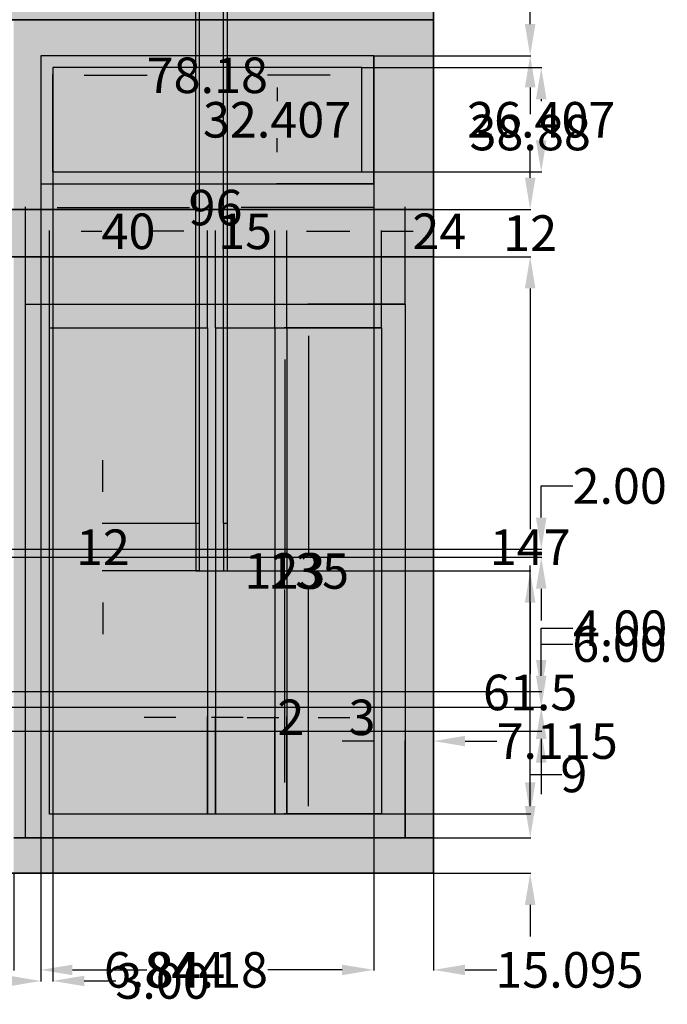
# Model space of a CAD drawing. Units: inches. Extents: x 207 to 609, y 30 to 576.
# Tile 2 of 4: x 445 to 609, y 30 to 279. Entities that reach past the tile are written whole.
import ezdxf

# ---------------------------------------------------------------- set-up
doc = ezdxf.new("R2010")
doc.units = ezdxf.units.IN
doc.header["$MEASUREMENT"] = 0
for name, color, linetype, lineweight in [('A-ANNO-DIMS', 2, 'Continuous', 18), ('A-DOOR', 3, 'Continuous', 25), ('A-ELEV', 7, 'Continuous', 35), ('A-ELEV-PATT', 251, 'Continuous', 13), ('A-ELEV-PATT-WOOD', 19, 'Continuous', 13), ('A-GLAZ', 4, 'Continuous', 25), ('A-GLAZ-PATT', 49, 'Continuous', 13)]:
    doc.layers.add(name, color=color, linetype=linetype, lineweight=lineweight)
doc.styles.get("Standard").update_dxf_attribs({"font": 'arial.ttf'})
doc.dimstyles.get("Standard").update_dxf_attribs({"dimtxt": 9, "dimasz": 8, "dimexe": 0.18, "dimexo": 0.0625, "dimgap": 0.09, "dimtad": 0, "dimtih": 1, "dimtoh": 1, "dimdec": 0, "dimzin": 0, "dimdsep": 46, "dimlunit": 3, "dimtxsty": 'Standard', "dimcen": 0.09, "dimadec": 0, "dimazin": 0, "dimtfac": 1, "dimtdec": 0, "dimtofl": 0, "dimtmove": 0, "dimatfit": 3, "dimfxl": 1, "dimtolj": 1, "dimtzin": 0, "dimarcsym": 0})

# ---------------------------------------------------------------- blocks, each defined once
blk = doc.blocks.new('*D18')
at = {"layer": 'A-ANNO-DIMS', "color": 0, "lineweight": -2, "transparency": 16777216}
for p, q in [((574.15, 79.79), (574.15, 87.79)), ((574.15, 87.79), (582.15, 87.79)), ((549.76, 71.79), (574.33, 71.79)), ((549.76, 62.79), (574.33, 62.79)), ((574.15, 54.79), (574.15, 46.79))]:
    blk.add_line(p, q, dxfattribs=at)
at = {"layer": 'A-ANNO-DIMS', "color": 0, "transparency": 16777216}
for points in [[(572.81, 79.79), (575.48, 79.79), (574.15, 71.79)], [(572.81, 54.79), (575.48, 54.79), (574.15, 62.79)]]:
    blk.add_solid(points, dxfattribs=at)
at = {"layer": 'Defpoints', "color": 0, "transparency": 16777216}
for p in [(549.7, 71.79), (574.15, 71.79), (549.7, 62.79)]:
    blk.add_point(p, dxfattribs=at)
at = {"layer": 'A-ANNO-DIMS', "color": 0, "transparency": 16777216, "insert": (585.19, 87.79), "char_height": 9, "attachment_point": 5}
blk.add_mtext('\\A1;9', dxfattribs=at)
blk = doc.blocks.new('*D19')
at = {"layer": 'A-ANNO-DIMS', "color": 0, "lineweight": -2, "transparency": 16777216}
for p, q in [((549.76, 218.79), (574.33, 218.79)), ((574.15, 210.79), (574.15, 149.89)), ((574.15, 79.79), (574.15, 140.68)), ((549.76, 71.79), (574.33, 71.79))]:
    blk.add_line(p, q, dxfattribs=at)
at = {"layer": 'A-ANNO-DIMS', "color": 0, "transparency": 16777216}
for points in [[(572.81, 210.79), (575.48, 210.79), (574.15, 218.79)], [(572.81, 79.79), (575.48, 79.79), (574.15, 71.79)]]:
    blk.add_solid(points, dxfattribs=at)
at = {"layer": 'Defpoints', "color": 0, "transparency": 16777216}
for p in [(549.7, 218.79), (574.15, 218.79), (549.7, 71.79)]:
    blk.add_point(p, dxfattribs=at)
at = {"layer": 'A-ANNO-DIMS', "color": 0, "transparency": 16777216, "insert": (574.15, 145.29), "char_height": 9, "attachment_point": 5}
blk.add_mtext('\\A1;147', dxfattribs=at)
blk = doc.blocks.new('*D20')
at = {"layer": 'A-ANNO-DIMS', "color": 0, "lineweight": -2, "transparency": 16777216}
for p, q in [((574.15, 238.79), (574.15, 246.79)), ((549.76, 230.79), (574.33, 230.79)), ((549.76, 218.79), (574.33, 218.79)), ((574.15, 210.79), (574.15, 202.79))]:
    blk.add_line(p, q, dxfattribs=at)
at = {"layer": 'A-ANNO-DIMS', "color": 0, "transparency": 16777216}
for points in [[(572.81, 238.79), (575.48, 238.79), (574.15, 230.79)], [(572.81, 210.79), (575.48, 210.79), (574.15, 218.79)]]:
    blk.add_solid(points, dxfattribs=at)
at = {"layer": 'Defpoints', "color": 0, "transparency": 16777216}
for p in [(549.7, 230.79), (574.15, 230.79), (549.7, 218.79)]:
    blk.add_point(p, dxfattribs=at)
at = {"layer": 'A-ANNO-DIMS', "color": 0, "transparency": 16777216, "insert": (574.15, 224.79), "char_height": 9, "attachment_point": 5}
blk.add_mtext('\\A1;12', dxfattribs=at)
blk = doc.blocks.new('*D21')
at = {"layer": 'A-ANNO-DIMS', "color": 0, "lineweight": -2, "transparency": 16777216}
for p, q in [((534.66, 269.66), (574.33, 269.66)), ((574.15, 261.66), (574.15, 254.91)), ((574.15, 238.79), (574.15, 245.54)), ((549.76, 230.79), (574.33, 230.79))]:
    blk.add_line(p, q, dxfattribs=at)
at = {"layer": 'A-ANNO-DIMS', "color": 0, "transparency": 16777216}
for points in [[(572.81, 261.66), (575.48, 261.66), (574.15, 269.66)], [(572.81, 238.79), (575.48, 238.79), (574.15, 230.79)]]:
    blk.add_solid(points, dxfattribs=at)
at = {"layer": 'Defpoints', "color": 0, "transparency": 16777216}
for p in [(534.6, 269.66), (574.15, 269.66), (549.7, 230.79)]:
    blk.add_point(p, dxfattribs=at)
at = {"layer": 'A-ANNO-DIMS', "color": 0, "transparency": 16777216, "insert": (574.15, 250.23), "char_height": 9, "attachment_point": 5}
blk.add_mtext('\\A1;38.88', dxfattribs=at)
blk = doc.blocks.new('*D22')
at = {"layer": 'A-ANNO-DIMS', "color": 0, "lineweight": -2, "transparency": 16777216}
for p, q in [((549.76, 302.79), (574.33, 302.79)), ((574.15, 294.79), (574.15, 290.91)), ((574.15, 277.66), (574.15, 281.54)), ((534.66, 269.66), (574.33, 269.66))]:
    blk.add_line(p, q, dxfattribs=at)
at = {"layer": 'A-ANNO-DIMS', "color": 0, "transparency": 16777216}
for points in [[(572.81, 294.79), (575.48, 294.79), (574.15, 302.79)], [(572.81, 277.66), (575.48, 277.66), (574.15, 269.66)]]:
    blk.add_solid(points, dxfattribs=at)
at = {"layer": 'Defpoints', "color": 0, "transparency": 16777216}
for p in [(549.7, 302.79), (574.15, 302.79), (534.6, 269.66)]:
    blk.add_point(p, dxfattribs=at)
at = {"layer": 'A-ANNO-DIMS', "color": 0, "transparency": 16777216, "insert": (574.15, 286.23), "char_height": 9, "attachment_point": 5}
blk.add_mtext('\\A1;33.12', dxfattribs=at)
blk = doc.blocks.new('*D32')
at = {"layer": 'A-ANNO-DIMS', "color": 0, "lineweight": -2, "transparency": 16777216}
for p, q in [((450.42, 269.6), (450.42, 38.16)), ((443.58, 62.72), (443.58, 38.16)), ((435.58, 38.34), (427.58, 38.34)), ((458.42, 38.34), (466.42, 38.34))]:
    blk.add_line(p, q, dxfattribs=at)
at = {"layer": 'A-ANNO-DIMS', "color": 0, "transparency": 16777216}
for points in [[(435.58, 39.67), (435.58, 37), (443.58, 38.34)], [(458.42, 39.67), (458.42, 37), (450.42, 38.34)]]:
    blk.add_solid(points, dxfattribs=at)
at = {"layer": 'Defpoints', "color": 0, "transparency": 16777216}
for p in [(450.42, 269.66), (443.58, 62.79), (450.42, 38.34)]:
    blk.add_point(p, dxfattribs=at)
at = {"layer": 'A-ANNO-DIMS', "color": 0, "transparency": 16777216, "insert": (481.71, 38.34), "char_height": 9, "attachment_point": 5}
blk.add_mtext('\\A1;6.844', dxfattribs=at)
blk = doc.blocks.new('*D33')
at = {"layer": 'A-ANNO-DIMS', "color": 0, "lineweight": -2, "transparency": 16777216}
for p, q in [((450.42, 269.6), (450.42, 38.16)), ((534.6, 269.6), (534.6, 38.16)), ((458.42, 38.34), (477.22, 38.34)), ((526.6, 38.34), (507.8, 38.34))]:
    blk.add_line(p, q, dxfattribs=at)
at = {"layer": 'A-ANNO-DIMS', "color": 0, "transparency": 16777216}
for points in [[(458.42, 39.67), (458.42, 37), (450.42, 38.34)], [(526.6, 39.67), (526.6, 37), (534.6, 38.34)]]:
    blk.add_solid(points, dxfattribs=at)
at = {"layer": 'Defpoints', "color": 0, "transparency": 16777216}
for p in [(450.42, 269.66), (534.6, 269.66), (534.6, 38.34)]:
    blk.add_point(p, dxfattribs=at)
at = {"layer": 'A-ANNO-DIMS', "color": 0, "transparency": 16777216, "insert": (492.51, 38.34), "char_height": 9, "attachment_point": 5}
blk.add_mtext('\\A1;84.18', dxfattribs=at)
blk = doc.blocks.new('*D34')
at = {"layer": 'A-ANNO-DIMS', "color": 0, "lineweight": -2, "transparency": 16777216}
for p, q in [((534.6, 269.6), (534.6, 38.16)), ((549.7, 62.72), (549.7, 38.16)), ((526.6, 38.34), (518.6, 38.34)), ((557.7, 38.34), (565.7, 38.34))]:
    blk.add_line(p, q, dxfattribs=at)
at = {"layer": 'A-ANNO-DIMS', "color": 0, "transparency": 16777216}
for points in [[(526.6, 39.67), (526.6, 37), (534.6, 38.34)], [(557.7, 39.67), (557.7, 37), (549.7, 38.34)]]:
    blk.add_solid(points, dxfattribs=at)
at = {"layer": 'Defpoints', "color": 0, "transparency": 16777216}
for p in [(534.6, 269.66), (549.7, 62.79), (549.7, 38.34)]:
    blk.add_point(p, dxfattribs=at)
at = {"layer": 'A-ANNO-DIMS', "color": 0, "transparency": 16777216, "insert": (584.08, 38.34), "char_height": 9, "attachment_point": 5}
blk.add_mtext('\\A1;15.095', dxfattribs=at)
blk = doc.blocks.new('*D35')
at = {"layer": 'A-ANNO-DIMS', "color": 0, "lineweight": -2, "transparency": 16777216}
for p, q in [((446.58, 206.85), (446.58, 231.42)), ((454.58, 231.24), (488.05, 231.24)), ((534.58, 231.24), (501.11, 231.24)), ((542.58, 206.85), (542.58, 231.42))]:
    blk.add_line(p, q, dxfattribs=at)
at = {"layer": 'A-ANNO-DIMS', "color": 0, "transparency": 16777216}
for points in [[(454.58, 232.57), (454.58, 229.9), (446.58, 231.24)], [(534.58, 232.57), (534.58, 229.9), (542.58, 231.24)]]:
    blk.add_solid(points, dxfattribs=at)
at = {"layer": 'Defpoints', "color": 0, "transparency": 16777216}
for p in [(542.58, 231.24), (446.58, 206.79), (542.58, 206.79)]:
    blk.add_point(p, dxfattribs=at)
at = {"layer": 'A-ANNO-DIMS', "color": 0, "transparency": 16777216, "insert": (494.58, 231.24), "char_height": 9, "attachment_point": 5}
blk.add_mtext('\\A1;96', dxfattribs=at)
blk = doc.blocks.new('*D36')
at = {"layer": 'A-ANNO-DIMS', "color": 0, "lineweight": -2, "transparency": 16777216}
for p, q in [((534.58, 96.24), (526.58, 96.24)), ((542.58, 71.85), (542.58, 96.42)), ((549.7, 71.85), (549.7, 96.42)), ((557.7, 96.24), (565.7, 96.24))]:
    blk.add_line(p, q, dxfattribs=at)
at = {"layer": 'A-ANNO-DIMS', "color": 0, "transparency": 16777216}
for points in [[(534.58, 97.57), (534.58, 94.9), (542.58, 96.24)], [(557.7, 97.57), (557.7, 94.9), (549.7, 96.24)]]:
    blk.add_solid(points, dxfattribs=at)
at = {"layer": 'Defpoints', "color": 0, "transparency": 16777216}
for p in [(549.7, 96.24), (542.58, 71.79), (549.7, 71.79)]:
    blk.add_point(p, dxfattribs=at)
at = {"layer": 'A-ANNO-DIMS', "color": 0, "transparency": 16777216, "insert": (580.97, 96.24), "char_height": 9, "attachment_point": 5}
blk.add_mtext('\\A1;7.115', dxfattribs=at)
blk = doc.blocks.new('*D37')
at = {"layer": 'A-ANNO-DIMS', "color": 0, "lineweight": -2, "transparency": 16777216}
for p, q in [((534.54, 269.66), (509.97, 269.66)), ((510.15, 261.66), (510.15, 258.15)), ((510.15, 245.26), (510.15, 248.77)), ((534.54, 237.26), (509.97, 237.26))]:
    blk.add_line(p, q, dxfattribs=at)
at = {"layer": 'A-ANNO-DIMS', "color": 0, "transparency": 16777216}
for points in [[(508.82, 261.66), (511.48, 261.66), (510.15, 269.66)], [(508.82, 245.26), (511.48, 245.26), (510.15, 237.26)]]:
    blk.add_solid(points, dxfattribs=at)
at = {"layer": 'Defpoints', "color": 0, "transparency": 16777216}
for p in [(510.15, 269.66), (534.6, 269.66), (534.6, 237.26)]:
    blk.add_point(p, dxfattribs=at)
at = {"layer": 'A-ANNO-DIMS', "color": 0, "transparency": 16777216, "insert": (510.15, 253.46), "char_height": 9, "attachment_point": 5}
blk.add_mtext('\\A1;32.407', dxfattribs=at)
blk = doc.blocks.new('*D38')
at = {"layer": 'A-ANNO-DIMS', "color": 0, "lineweight": -2, "transparency": 16777216}
for p, q in [((453.42, 240.32), (453.42, 264.89)), ((461.42, 264.71), (477.27, 264.71)), ((523.6, 264.71), (507.76, 264.71)), ((531.6, 240.32), (531.6, 264.89))]:
    blk.add_line(p, q, dxfattribs=at)
at = {"layer": 'A-ANNO-DIMS', "color": 0, "transparency": 16777216}
for points in [[(461.42, 266.04), (461.42, 263.37), (453.42, 264.71)], [(523.6, 266.04), (523.6, 263.37), (531.6, 264.71)]]:
    blk.add_solid(points, dxfattribs=at)
at = {"layer": 'Defpoints', "color": 0, "transparency": 16777216}
for p in [(531.6, 264.71), (453.42, 240.26), (531.6, 240.26)]:
    blk.add_point(p, dxfattribs=at)
at = {"layer": 'A-ANNO-DIMS', "color": 0, "transparency": 16777216, "insert": (492.51, 264.71), "char_height": 9, "attachment_point": 5}
blk.add_mtext('\\A1;78.18', dxfattribs=at)
blk = doc.blocks.new('*D62')
at = {"layer": 'A-ANNO-DIMS', "color": 0, "lineweight": -2, "transparency": 16777216}
for p, q in [((452.58, 200.85), (452.58, 225.42)), ((460.58, 225.24), (465.88, 225.24)), ((484.58, 225.24), (479.28, 225.24)), ((492.58, 200.85), (492.58, 225.42))]:
    blk.add_line(p, q, dxfattribs=at)
at = {"layer": 'A-ANNO-DIMS', "color": 0, "transparency": 16777216}
for points in [[(460.58, 226.57), (460.58, 223.9), (452.58, 225.24)], [(484.58, 226.57), (484.58, 223.9), (492.58, 225.24)]]:
    blk.add_solid(points, dxfattribs=at)
at = {"layer": 'Defpoints', "color": 0, "transparency": 16777216}
for p in [(492.58, 225.24), (452.58, 200.79), (492.58, 200.79)]:
    blk.add_point(p, dxfattribs=at)
at = {"layer": 'A-ANNO-DIMS', "color": 0, "transparency": 16777216, "insert": (472.58, 225.24), "char_height": 9, "attachment_point": 5}
blk.add_mtext('\\A1;40', dxfattribs=at)
blk = doc.blocks.new('*D63')
at = {"layer": 'A-ANNO-DIMS', "color": 0, "lineweight": -2, "transparency": 16777216}
for p, q in [((486.58, 225.24), (478.58, 225.24)), ((494.58, 200.85), (494.58, 225.42)), ((509.58, 200.85), (509.58, 225.42)), ((517.58, 225.24), (525.58, 225.24))]:
    blk.add_line(p, q, dxfattribs=at)
at = {"layer": 'A-ANNO-DIMS', "color": 0, "transparency": 16777216}
for points in [[(486.58, 226.57), (486.58, 223.9), (494.58, 225.24)], [(517.58, 226.57), (517.58, 223.9), (509.58, 225.24)]]:
    blk.add_solid(points, dxfattribs=at)
at = {"layer": 'Defpoints', "color": 0, "transparency": 16777216}
for p in [(509.58, 225.24), (494.58, 200.79), (509.58, 200.79)]:
    blk.add_point(p, dxfattribs=at)
at = {"layer": 'A-ANNO-DIMS', "color": 0, "transparency": 16777216, "insert": (502.08, 225.24), "char_height": 9, "attachment_point": 5}
blk.add_mtext('\\A1;15', dxfattribs=at)
blk = doc.blocks.new('*D64')
at = {"layer": 'A-ANNO-DIMS', "color": 0, "lineweight": -2, "transparency": 16777216}
for p, q in [((512.58, 200.85), (512.58, 225.42)), ((520.58, 225.24), (528.58, 225.24)), ((536.58, 200.85), (536.58, 225.42)), ((536.58, 225.24), (544.58, 225.24))]:
    blk.add_line(p, q, dxfattribs=at)
at = {"layer": 'A-ANNO-DIMS', "color": 0, "transparency": 16777216}
for points in [[(520.58, 226.57), (520.58, 223.9), (512.58, 225.24)], [(528.58, 226.57), (528.58, 223.9), (536.58, 225.24)]]:
    blk.add_solid(points, dxfattribs=at)
at = {"layer": 'Defpoints', "color": 0, "transparency": 16777216}
for p in [(536.58, 225.24), (512.58, 200.79), (536.58, 200.79)]:
    blk.add_point(p, dxfattribs=at)
at = {"layer": 'A-ANNO-DIMS', "color": 0, "transparency": 16777216, "insert": (551.18, 225.24), "char_height": 9, "attachment_point": 5}
blk.add_mtext('\\A1;24', dxfattribs=at)
blk = doc.blocks.new('*D65')
at = {"layer": 'A-ANNO-DIMS', "color": 0, "lineweight": -2, "transparency": 16777216}
for p, q in [((484.58, 102.24), (476.58, 102.24)), ((492.58, 77.85), (492.58, 102.42)), ((494.58, 77.85), (494.58, 102.42)), ((502.58, 102.24), (510.58, 102.24))]:
    blk.add_line(p, q, dxfattribs=at)
at = {"layer": 'A-ANNO-DIMS', "color": 0, "transparency": 16777216}
for points in [[(484.58, 103.57), (484.58, 100.9), (492.58, 102.24)], [(502.58, 103.57), (502.58, 100.9), (494.58, 102.24)]]:
    blk.add_solid(points, dxfattribs=at)
at = {"layer": 'Defpoints', "color": 0, "transparency": 16777216}
for p in [(494.58, 102.24), (492.58, 77.79), (494.58, 77.79)]:
    blk.add_point(p, dxfattribs=at)
at = {"layer": 'A-ANNO-DIMS', "color": 0, "transparency": 16777216, "insert": (513.65, 102.24), "char_height": 9, "attachment_point": 5}
blk.add_mtext('\\A1;2', dxfattribs=at)
blk = doc.blocks.new('*D66')
at = {"layer": 'A-ANNO-DIMS', "color": 0, "lineweight": -2, "transparency": 16777216}
for p, q in [((501.58, 102.24), (493.58, 102.24)), ((509.58, 77.85), (509.58, 102.42)), ((512.58, 77.85), (512.58, 102.42)), ((520.58, 102.24), (528.58, 102.24))]:
    blk.add_line(p, q, dxfattribs=at)
at = {"layer": 'A-ANNO-DIMS', "color": 0, "transparency": 16777216}
for points in [[(501.58, 103.57), (501.58, 100.9), (509.58, 102.24)], [(520.58, 103.57), (520.58, 100.9), (512.58, 102.24)]]:
    blk.add_solid(points, dxfattribs=at)
at = {"layer": 'Defpoints', "color": 0, "transparency": 16777216}
for p in [(512.58, 102.24), (509.58, 77.79), (512.58, 77.79)]:
    blk.add_point(p, dxfattribs=at)
at = {"layer": 'A-ANNO-DIMS', "color": 0, "transparency": 16777216, "insert": (531.62, 102.24), "char_height": 9, "attachment_point": 5}
blk.add_mtext('\\A1;3', dxfattribs=at)
blk = doc.blocks.new('*D67')
at = {"layer": 'A-ANNO-DIMS', "color": 0, "lineweight": -2, "transparency": 16777216}
for p, q in [((542.52, 206.79), (517.95, 206.79)), ((518.13, 198.79), (518.13, 143.97)), ((518.13, 79.79), (518.13, 134.6)), ((542.52, 71.79), (517.95, 71.79))]:
    blk.add_line(p, q, dxfattribs=at)
at = {"layer": 'A-ANNO-DIMS', "color": 0, "transparency": 16777216}
for points in [[(516.8, 198.79), (519.46, 198.79), (518.13, 206.79)], [(516.8, 79.79), (519.46, 79.79), (518.13, 71.79)]]:
    blk.add_solid(points, dxfattribs=at)
at = {"layer": 'Defpoints', "color": 0, "transparency": 16777216}
for p in [(518.13, 206.79), (542.58, 206.79), (542.58, 71.79)]:
    blk.add_point(p, dxfattribs=at)
at = {"layer": 'A-ANNO-DIMS', "color": 0, "transparency": 16777216, "insert": (518.13, 139.29), "char_height": 9, "attachment_point": 5}
blk.add_mtext('\\A1;135', dxfattribs=at)
blk = doc.blocks.new('*D68')
at = {"layer": 'A-ANNO-DIMS', "color": 0, "lineweight": -2, "transparency": 16777216}
for p, q in [((536.52, 200.79), (511.95, 200.79)), ((512.13, 192.79), (512.13, 143.97)), ((512.13, 85.79), (512.13, 134.6)), ((536.52, 77.79), (511.95, 77.79))]:
    blk.add_line(p, q, dxfattribs=at)
at = {"layer": 'A-ANNO-DIMS', "color": 0, "transparency": 16777216}
for points in [[(510.8, 192.79), (513.46, 192.79), (512.13, 200.79)], [(510.8, 85.79), (513.46, 85.79), (512.13, 77.79)]]:
    blk.add_solid(points, dxfattribs=at)
at = {"layer": 'Defpoints', "color": 0, "transparency": 16777216}
for p in [(512.13, 200.79), (536.58, 200.79), (536.58, 77.79)]:
    blk.add_point(p, dxfattribs=at)
at = {"layer": 'A-ANNO-DIMS', "color": 0, "transparency": 16777216, "insert": (512.13, 139.29), "char_height": 9, "attachment_point": 5}
blk.add_mtext('\\A1;123', dxfattribs=at)
blk = doc.blocks.new('*D69')
at = {"layer": 'A-ANNO-DIMS', "color": 0, "lineweight": -2, "transparency": 16777216}
for p, q in [((490.64, 139.29), (574.33, 139.29)), ((574.15, 131.29), (574.15, 113.22)), ((574.15, 85.79), (574.15, 103.85)), ((492.64, 77.79), (574.33, 77.79))]:
    blk.add_line(p, q, dxfattribs=at)
at = {"layer": 'A-ANNO-DIMS', "color": 0, "transparency": 16777216}
for points in [[(572.81, 131.29), (575.48, 131.29), (574.15, 139.29)], [(572.81, 85.79), (575.48, 85.79), (574.15, 77.79)]]:
    blk.add_solid(points, dxfattribs=at)
at = {"layer": 'Defpoints', "color": 0, "transparency": 16777216}
for p in [(490.58, 139.29), (574.15, 139.29), (492.58, 77.79)]:
    blk.add_point(p, dxfattribs=at)
at = {"layer": 'A-ANNO-DIMS', "color": 0, "transparency": 16777216, "insert": (574.15, 108.54), "char_height": 9, "attachment_point": 5}
blk.add_mtext('\\A1;61.5', dxfattribs=at)
blk = doc.blocks.new('*D70')
at = {"layer": 'A-ANNO-DIMS', "color": 0, "lineweight": -2, "transparency": 16777216}
for p, q in [((466.13, 159.29), (466.13, 167.29)), ((490.52, 151.29), (465.95, 151.29)), ((490.52, 139.29), (465.95, 139.29)), ((466.13, 131.29), (466.13, 123.29))]:
    blk.add_line(p, q, dxfattribs=at)
at = {"layer": 'A-ANNO-DIMS', "color": 0, "transparency": 16777216}
for points in [[(464.8, 159.29), (467.46, 159.29), (466.13, 151.29)], [(464.8, 131.29), (467.46, 131.29), (466.13, 139.29)]]:
    blk.add_solid(points, dxfattribs=at)
at = {"layer": 'Defpoints', "color": 0, "transparency": 16777216}
for p in [(466.13, 151.29), (490.58, 151.29), (490.58, 139.29)]:
    blk.add_point(p, dxfattribs=at)
at = {"layer": 'A-ANNO-DIMS', "color": 0, "transparency": 16777216, "insert": (466.13, 145.29), "char_height": 9, "attachment_point": 5}
blk.add_mtext('\\A1;12', dxfattribs=at)
blk = doc.blocks.new('*D75')
at = {"layer": 'A-ANNO-DIMS', "color": 0, "lineweight": -2, "transparency": 16777216}
for p, q in [((576.95, 112.79), (576.95, 120.79)), ((576.95, 120.79), (584.95, 120.79)), ((355.76, 104.79), (577.13, 104.79)), ((361.76, 98.79), (577.13, 98.79)), ((576.95, 90.79), (576.95, 82.79))]:
    blk.add_line(p, q, dxfattribs=at)
at = {"layer": 'A-ANNO-DIMS', "color": 0, "transparency": 16777216}
for points in [[(575.61, 112.79), (578.28, 112.79), (576.95, 104.79)], [(575.61, 90.79), (578.28, 90.79), (576.95, 98.79)]]:
    blk.add_solid(points, dxfattribs=at)
at = {"layer": 'Defpoints', "color": 0, "transparency": 16777216}
for p in [(355.7, 104.79), (576.95, 104.79), (361.7, 98.79)]:
    blk.add_point(p, dxfattribs=at)
at = {"layer": 'A-ANNO-DIMS', "color": 0, "transparency": 16777216, "insert": (596.73, 120.79), "char_height": 9, "attachment_point": 5}
blk.add_mtext('\\A1;6.00', dxfattribs=at)
blk = doc.blocks.new('*D76')
at = {"layer": 'A-ANNO-DIMS', "color": 0, "lineweight": -2, "transparency": 16777216}
for p, q in [((576.95, 116.79), (576.95, 124.79)), ((576.95, 124.79), (584.95, 124.79)), ((351.76, 108.79), (577.13, 108.79)), ((355.76, 104.79), (577.13, 104.79)), ((576.95, 96.79), (576.95, 88.79))]:
    blk.add_line(p, q, dxfattribs=at)
at = {"layer": 'A-ANNO-DIMS', "color": 0, "transparency": 16777216}
for points in [[(575.61, 116.79), (578.28, 116.79), (576.95, 108.79)], [(575.61, 96.79), (578.28, 96.79), (576.95, 104.79)]]:
    blk.add_solid(points, dxfattribs=at)
at = {"layer": 'Defpoints', "color": 0, "transparency": 16777216}
for p in [(351.7, 108.79), (576.95, 108.79), (355.7, 104.79)]:
    blk.add_point(p, dxfattribs=at)
at = {"layer": 'A-ANNO-DIMS', "color": 0, "transparency": 16777216, "insert": (596.89, 124.79), "char_height": 9, "attachment_point": 5}
blk.add_mtext('\\A1;4.00', dxfattribs=at)
blk = doc.blocks.new('*D77')
at = {"layer": 'A-ANNO-DIMS', "color": 0, "lineweight": -2, "transparency": 16777216}
for p, q in [((576.95, 152.79), (576.95, 160.79)), ((576.95, 160.79), (584.95, 160.79)), ((351.76, 144.79), (577.13, 144.79)), ((351.76, 142.79), (577.13, 142.79)), ((576.95, 134.79), (576.95, 126.79))]:
    blk.add_line(p, q, dxfattribs=at)
at = {"layer": 'A-ANNO-DIMS', "color": 0, "transparency": 16777216}
for points in [[(575.61, 152.79), (578.28, 152.79), (576.95, 144.79)], [(575.61, 134.79), (578.28, 134.79), (576.95, 142.79)]]:
    blk.add_solid(points, dxfattribs=at)
at = {"layer": 'Defpoints', "color": 0, "transparency": 16777216}
for p in [(351.7, 144.79), (576.95, 144.79), (351.7, 142.79)]:
    blk.add_point(p, dxfattribs=at)
at = {"layer": 'A-ANNO-DIMS', "color": 0, "transparency": 16777216, "insert": (596.79, 160.79), "char_height": 9, "attachment_point": 5}
blk.add_mtext('\\A1;2.00', dxfattribs=at)
blk = doc.blocks.new('*D79')
at = {"layer": 'A-ANNO-DIMS', "color": 0, "lineweight": -2, "transparency": 16777216}
for p, q in [((453.42, 240.19), (453.42, 35.36)), ((450.42, 237.19), (450.42, 35.36)), ((442.42, 35.54), (434.42, 35.54)), ((461.42, 35.54), (469.42, 35.54))]:
    blk.add_line(p, q, dxfattribs=at)
at = {"layer": 'A-ANNO-DIMS', "color": 0, "transparency": 16777216}
for points in [[(442.42, 36.87), (442.42, 34.2), (450.42, 35.54)], [(461.42, 36.87), (461.42, 34.2), (453.42, 35.54)]]:
    blk.add_solid(points, dxfattribs=at)
at = {"layer": 'Defpoints', "color": 0, "transparency": 16777216}
for p in [(453.42, 240.26), (450.42, 237.26), (453.42, 35.54)]:
    blk.add_point(p, dxfattribs=at)
at = {"layer": 'A-ANNO-DIMS', "color": 0, "transparency": 16777216, "insert": (481.19, 35.54), "char_height": 9, "attachment_point": 5}
blk.add_mtext('\\A1;3.00', dxfattribs=at)
blk = doc.blocks.new('*D80')
at = {"layer": 'A-ANNO-DIMS', "color": 0, "lineweight": -2, "transparency": 16777216}
for p, q in [((531.66, 266.66), (577.13, 266.66)), ((576.95, 258.66), (576.95, 258.15)), ((576.95, 248.26), (576.95, 248.78)), ((531.66, 240.26), (577.13, 240.26))]:
    blk.add_line(p, q, dxfattribs=at)
at = {"layer": 'A-ANNO-DIMS', "color": 0, "transparency": 16777216}
for points in [[(575.61, 258.66), (578.28, 258.66), (576.95, 266.66)], [(575.61, 248.26), (578.28, 248.26), (576.95, 240.26)]]:
    blk.add_solid(points, dxfattribs=at)
at = {"layer": 'Defpoints', "color": 0, "transparency": 16777216}
for p in [(531.6, 266.66), (576.95, 266.66), (531.6, 240.26)]:
    blk.add_point(p, dxfattribs=at)
at = {"layer": 'A-ANNO-DIMS', "color": 0, "transparency": 16777216, "insert": (576.95, 253.46), "char_height": 9, "attachment_point": 5}
blk.add_mtext('\\A1;26.407', dxfattribs=at)
blk = doc.blocks.new('*D81')
at = {"layer": 'A-ANNO-DIMS', "color": 0, "lineweight": -2, "transparency": 16777216}
for p, q in [((481.58, 570.04), (473.58, 570.04)), ((489.58, 151.35), (489.58, 570.22)), ((490.58, 151.35), (490.58, 570.22)), ((498.58, 570.04), (506.58, 570.04))]:
    blk.add_line(p, q, dxfattribs=at)
at = {"layer": 'A-ANNO-DIMS', "color": 0, "transparency": 16777216}
for points in [[(481.58, 571.37), (481.58, 568.7), (489.58, 570.04)], [(498.58, 571.37), (498.58, 568.7), (490.58, 570.04)]]:
    blk.add_solid(points, dxfattribs=at)
at = {"layer": 'Defpoints', "color": 0, "transparency": 16777216}
for p in [(490.58, 570.04), (489.58, 151.29), (490.58, 151.29)]:
    blk.add_point(p, dxfattribs=at)
at = {"layer": 'A-ANNO-DIMS', "color": 0, "transparency": 16777216, "insert": (517.92, 570.04), "char_height": 9, "attachment_point": 5}
blk.add_mtext('\\A1;1.00', dxfattribs=at)
blk = doc.blocks.new('*D82')
at = {"layer": 'A-ANNO-DIMS', "color": 0, "lineweight": -2, "transparency": 16777216}
for p, q in [((488.58, 570.04), (480.58, 570.04)), ((496.58, 151.35), (496.58, 570.22)), ((497.58, 151.35), (497.58, 570.22)), ((505.58, 570.04), (513.58, 570.04))]:
    blk.add_line(p, q, dxfattribs=at)
at = {"layer": 'A-ANNO-DIMS', "color": 0, "transparency": 16777216}
for points in [[(488.58, 571.37), (488.58, 568.7), (496.58, 570.04)], [(505.58, 571.37), (505.58, 568.7), (497.58, 570.04)]]:
    blk.add_solid(points, dxfattribs=at)
at = {"layer": 'Defpoints', "color": 0, "transparency": 16777216}
for p in [(497.58, 570.04), (496.58, 151.29), (497.58, 151.29)]:
    blk.add_point(p, dxfattribs=at)
at = {"layer": 'A-ANNO-DIMS', "color": 0, "transparency": 16777216, "insert": (524.92, 570.04), "char_height": 9, "attachment_point": 5}
blk.add_mtext('\\A1;1.00', dxfattribs=at)

msp = doc.modelspace()

# ---------------------------------------------------------------- hatches: boundary and pattern name
at = {"layer": 'A-ELEV-PATT'}
h = msp.add_hatch(color=256, dxfattribs=at)
h.dxf.hatch_style = 1
h.paths.add_polyline_path([(549.6956, 542.7864), (443.656, 542.7864), (443.656, 470.7864), (549.6956, 470.7864)])
h.paths.add_polyline_path([(549.6956, 230.7864), (249.6956, 230.7864), (249.6956, 218.7864), (549.6956, 218.7864)])
h.paths.add_polyline_path([(377.5808, 80.7864), (265.6956, 80.7864), (265.6956, 62.7864), (377.5808, 62.7864)])
h.paths.add_polyline_path([(549.6956, 71.7864), (443.5808, 71.7864), (443.5808, 62.7864), (549.6956, 62.7864)])
h = msp.add_hatch(color=256, dxfattribs=at)
h.dxf.hatch_style = 1
h.paths.add_polyline_path([(549.6956, 470.7864), (309.6956, 470.7864), (309.6956, 278.7864), (549.6956, 278.7864), (549.6956, 302.7864), (324.6956, 302.7864), (324.6956, 455.7864), (549.6956, 455.7864)])
h = msp.add_hatch(color=256, dxfattribs=at)
h.dxf.hatch_style = 1
h.paths.add_polyline_path([(265.6956, 302.7864), (249.6956, 302.7864), (249.6956, 230.7864), (265.6956, 230.7864)])
h.paths.add_polyline_path([(265.6956, 218.7864), (249.6956, 218.7864), (249.6956, 62.7864), (265.6956, 62.7864)])
h.paths.add_polyline_path([(549.6956, 278.7864), (443.5808, 278.7864), (443.5808, 230.7864), (549.6956, 230.7864)])
h.paths.add_polyline_path([(534.6005, 237.2568), (450.425, 237.2568), (450.425, 269.6636), (534.6005, 269.6636)], flags=16)
h.paths.add_polyline_path([(531.6005, 240.2568), (453.425, 240.2568), (453.425, 266.6636), (531.6005, 266.6636)], flags=0)
at = {"layer": 'A-ELEV-PATT', "transparency": 33554656}
msp.add_hatch(color=256, dxfattribs=at).paths.add_polyline_path([(549.6956, 218.7864), (443.5808, 218.7864), (443.5808, 71.7864), (446.5808, 71.7864), (446.5808, 206.7864), (542.5808, 206.7864), (542.5808, 71.7864), (549.6956, 71.7864)])
at = {"layer": 'A-ELEV-PATT-WOOD', "transparency": 33554656}
h = msp.add_hatch(color=256, dxfattribs=at)
h.paths.add_polyline_path([(490.5808, 151.2864), (489.5808, 151.2864), (489.5808, 139.2864), (490.5808, 139.2864)])
h.paths.add_polyline_path([(497.5808, 151.2864), (496.5808, 151.2864), (496.5808, 139.2864), (497.5808, 139.2864)])
h.paths.add_polyline_path([(499.8522, 371.716), (498.6956, 371.716), (498.6956, 359.7864), (499.8522, 359.7864)])
h = msp.add_hatch(color=256, dxfattribs=at)
h.paths.add_polyline_path([(450.425, 269.6636), (450.425, 237.2568), (534.6005, 237.2568), (534.6005, 269.6636)])
h.paths.add_polyline_path([(531.6005, 266.6636), (531.6005, 240.2568), (453.425, 240.2568), (453.425, 266.6636)], flags=16)
h.paths.add_polyline_path([(446.5808, 206.7864), (446.5808, 71.7864), (542.5808, 71.7864), (542.5808, 206.7864)])
h.paths.add_polyline_path([(512.5808, 200.7864), (536.5808, 200.7864), (536.5808, 77.7864), (512.5808, 77.7864)], flags=16)
h.paths.add_polyline_path([(355.6956, 196.7864), (287.6956, 196.7864), (287.6956, 104.7864), (355.6956, 104.7864)])
h.paths.add_polyline_path([(319.6956, 192.7864), (319.6956, 158.7864), (291.6956, 158.7864), (291.6956, 192.7864)], flags=16)
h.paths.add_polyline_path([(323.6956, 192.7864), (351.6956, 192.7864), (351.6956, 158.7864), (323.6956, 158.7864)], flags=16)
h.paths.add_polyline_path([(319.6956, 156.7864), (319.6956, 144.7864), (291.6956, 144.7864), (291.6956, 156.7864)], flags=16)
h.paths.add_polyline_path([(323.6956, 156.7864), (351.6956, 156.7864), (351.6956, 144.7864), (323.6956, 144.7864)], flags=16)
h.paths.add_polyline_path([(319.6956, 142.7864), (319.6956, 108.7864), (291.6956, 108.7864), (291.6956, 142.7864)], flags=16)
h.paths.add_polyline_path([(323.6956, 142.7864), (351.6956, 142.7864), (351.6956, 108.7864), (323.6956, 108.7864)], flags=16)
h.paths.add_polyline_path([(496.5808, 139.2864), (497.5808, 139.2864), (497.5808, 151.2864), (496.5808, 151.2864)], flags=16)
h.paths.add_polyline_path([(490.5808, 151.2864), (489.5808, 151.2864), (489.5808, 139.2864), (490.5808, 139.2864)], flags=0)
h = msp.add_hatch(color=256, dxfattribs=at)
h.paths.add_polyline_path([(531.6005, 266.6636), (453.425, 266.6636), (453.425, 240.2568), (531.6005, 240.2568)])
h.paths.add_polyline_path([(351.6956, 192.7864), (323.6956, 192.7864), (323.6956, 158.7864), (351.6956, 158.7864)])
h.paths.add_polyline_path([(319.6956, 192.7864), (291.6956, 192.7864), (291.6956, 158.7864), (319.6956, 158.7864)])
h.paths.add_polyline_path([(319.6956, 156.7864), (291.6956, 156.7864), (291.6956, 144.7864), (319.6956, 144.7864)])
h.paths.add_polyline_path([(351.6956, 156.7864), (323.6956, 156.7864), (323.6956, 144.7864), (351.6956, 144.7864)])
h.paths.add_polyline_path([(351.6956, 142.7864), (323.6956, 142.7864), (323.6956, 108.7864), (351.6956, 108.7864)])
h.paths.add_polyline_path([(319.6956, 142.7864), (291.6956, 142.7864), (291.6956, 108.7864), (319.6956, 108.7864)])
h.paths.add_polyline_path([(536.5808, 200.7864), (512.5808, 200.7864), (512.5808, 77.7864), (536.5808, 77.7864)])
msp.add_hatch(color=256, dxfattribs=at).paths.add_polyline_path([(492.5808, 77.7864), (494.5808, 77.7864), (494.5808, 200.7864), (492.5808, 200.7864)])
at = {"layer": 'A-GLAZ-PATT', "transparency": 33554656}
h = msp.add_hatch(color=256, dxfattribs=at)
h.paths.add_polyline_path([(489.5808, 151.2864), (490.5808, 151.2864), (490.5808, 139.2864), (489.5808, 139.2864)], flags=16)
h.paths.add_polyline_path([(497.5808, 151.2864), (497.5808, 139.2864), (496.5808, 139.2864), (496.5808, 151.2864)], flags=16)
h.paths.add_polyline_path([(492.5808, 200.7864), (452.5808, 200.7864), (452.5808, 77.7864), (492.5808, 77.7864)])
h.paths.add_polyline_path([(509.5808, 200.7864), (494.5808, 200.7864), (494.5808, 77.7864), (509.5808, 77.7864)])

# ---------------------------------------------------------------- linework, layer by layer
at = {"layer": 'A-DOOR'}
for p, q in [((452.5808, 200.7864), (492.5808, 200.7864)), ((452.5808, 77.7864), (452.5808, 200.7864)), ((492.5808, 200.7864), (492.5808, 77.7864)), ((494.5808, 200.7864), (494.5808, 77.7864)), ((494.5808, 200.7864), (512.5808, 200.7864)), ((509.5808, 200.7864), (509.5808, 77.7864)), ((512.5808, 200.7864), (512.5808, 77.7864)), ((512.5808, 200.7864), (536.5808, 200.7864)), ((536.5808, 200.7864), (536.5808, 77.7864)), ((492.5808, 77.7864), (452.5808, 77.7864)), ((509.5808, 77.7864), (494.5808, 77.7864)), ((536.5808, 77.7864), (512.5808, 77.7864))]:
    msp.add_line(p, q, dxfattribs=at)
for points in [[(446.5808, 206.7864), (542.5808, 206.7864), (542.5808, 71.7864), (446.5808, 71.7864)], [(489.5808, 139.2864), (490.5808, 139.2864), (490.5808, 151.2864), (489.5808, 151.2864)], [(496.5808, 139.2864), (497.5808, 139.2864), (497.5808, 151.2864), (496.5808, 151.2864)]]:
    msp.add_lwpolyline(points, close=True, dxfattribs=at)
at = {"layer": 'A-ELEV'}
for p, q in [((549.6956, 542.7864), (549.6956, 62.7864)), ((549.6956, 278.7864), (309.6956, 278.7864)), ((549.6956, 230.7864), (249.6956, 230.7864)), ((549.6956, 218.7864), (249.6956, 218.7864)), ((549.6956, 71.7864), (443.5808, 71.7864)), ((549.6956, 62.7864), (249.6956, 62.7864))]:
    msp.add_line(p, q, dxfattribs=at)
at = {"layer": 'A-GLAZ'}
for points in [[(450.425, 237.2568), (534.6005, 237.2568), (534.6005, 269.6636), (450.425, 269.6636)], [(453.425, 240.2568), (531.6005, 240.2568), (531.6005, 266.6636), (453.425, 266.6636)]]:
    msp.add_lwpolyline(points, close=True, dxfattribs=at)

# ---------------------------------------------------------------- dimensions: what is measured, and where the dimension line sits
at = {"layer": 'A-ANNO-DIMS'}
for base, p1, p2, override, picture, middle in [((490.5808, 570.0364), (489.5808, 151.2864), (490.5808, 151.2864), {"dimdec": 2, "dimlfac": 1, "dimrnd": 0, "dimzin": 0, "dimdsep": 46, "dimlunit": 2}, '*D81', (517.9208, 570.0364)), ((497.5808, 570.0364), (496.5808, 151.2864), (497.5808, 151.2864), {"dimdec": 2, "dimlfac": 1, "dimrnd": 0, "dimzin": 0, "dimdsep": 46, "dimlunit": 2}, '*D82', (524.9208, 570.0364)), ((450.425, 38.3364), (443.5808, 62.7864), (450.425, 269.6636), {"dimdec": 3, "dimlfac": 1, "dimrnd": 0, "dimzin": 0, "dimdsep": 46, "dimlunit": 2}, '*D32', (481.7063, 38.3364)), ((534.6005, 38.3364), (450.425, 269.6636), (534.6005, 269.6636), {"dimdec": 2, "dimlfac": 1, "dimrnd": 0, "dimzin": 0, "dimdsep": 46, "dimlunit": 2}, '*D33', (492.5127, 38.3364)), ((531.6005, 264.7068), (453.425, 240.2568), (531.6005, 240.2568), {"dimdec": 2, "dimlfac": 1, "dimrnd": 0, "dimzin": 0, "dimdsep": 46, "dimlunit": 2}, '*D38', (492.5127, 264.7068)), ((549.6956, 38.3364), (534.6005, 269.6636), (549.6956, 62.7864), {"dimdec": 3, "dimlfac": 1, "dimrnd": 0, "dimzin": 0, "dimdsep": 46, "dimlunit": 2}, '*D34', (584.0772, 38.3364)), ((453.425, 35.5364), (450.425, 237.2568), (453.425, 240.2568), {"dimdec": 2, "dimlfac": 1, "dimrnd": 0, "dimzin": 0, "dimdsep": 46, "dimlunit": 2}, '*D79', (481.1855, 35.5364)), ((542.5808, 231.2364), (446.5808, 206.7864), (542.5808, 206.7864), {"dimdec": 0, "dimlfac": 1, "dimrnd": 0, "dimzin": 0, "dimdsep": 46, "dimlunit": 2}, '*D35', (494.5808, 231.2364)), ((492.5808, 225.2364), (452.5808, 200.7864), (492.5808, 200.7864), {"dimdec": 0, "dimlfac": 1, "dimrnd": 0, "dimzin": 0, "dimdsep": 46, "dimlunit": 2}, '*D62', (472.5808, 225.2364)), ((509.5808, 225.2364), (494.5808, 200.7864), (509.5808, 200.7864), {"dimdec": 0, "dimlfac": 1, "dimrnd": 0, "dimzin": 0, "dimdsep": 46, "dimlunit": 2}, '*D63', (502.0808, 225.2364)), ((536.5808, 225.2364), (512.5808, 200.7864), (536.5808, 200.7864), {"dimdec": 0, "dimlfac": 1, "dimrnd": 0, "dimzin": 0, "dimdsep": 46, "dimlunit": 2}, '*D64', (551.1752, 225.2364)), ((494.5808, 102.2364), (492.5808, 77.7864), (494.5808, 77.7864), {"dimdec": 0, "dimlfac": 1, "dimrnd": 0, "dimzin": 0, "dimdsep": 46, "dimlunit": 2}, '*D65', (513.6513, 102.2364)), ((512.5808, 102.2364), (509.5808, 77.7864), (512.5808, 77.7864), {"dimdec": 0, "dimlfac": 1, "dimrnd": 0, "dimzin": 0, "dimdsep": 46, "dimlunit": 2}, '*D66', (531.6176, 102.2364)), ((549.6956, 96.2364), (542.5808, 71.7864), (549.6956, 71.7864), {"dimdec": 3, "dimlfac": 1, "dimrnd": 0, "dimzin": 0, "dimdsep": 46, "dimlunit": 2}, '*D36', (580.9677, 96.2364))]:
    dim = msp.add_linear_dim(base=base, p1=p1, p2=p2, dimstyle='Standard', override=override, dxfattribs=at)
    dim.commit()
    dim.dimension.update_dxf_attribs({"geometry": picture, "text_midpoint": middle})
for base, p1, p2, override, picture, middle in [((574.1456, 302.7864), (534.6005, 269.6636), (549.6956, 302.7864), {"dimdec": 2, "dimlfac": 1, "dimrnd": 0, "dimzin": 0, "dimdsep": 46, "dimlunit": 2}, '*D22', (574.1456, 286.225)), ((510.1505, 269.6636), (534.6005, 237.2568), (534.6005, 269.6636), {"dimdec": 3, "dimlfac": 1, "dimrnd": 0, "dimzin": 0, "dimdsep": 46, "dimlunit": 2}, '*D37', (510.1505, 253.4602)), ((574.1456, 269.6636), (549.6956, 230.7864), (534.6005, 269.6636), {"dimdec": 2, "dimlfac": 1, "dimrnd": 0, "dimzin": 0, "dimdsep": 46, "dimlunit": 2}, '*D21', (574.1456, 250.225)), ((576.9456, 266.6636), (531.6005, 240.2568), (531.6005, 266.6636), {"dimdec": 3, "dimlfac": 1, "dimrnd": 0, "dimzin": 0, "dimdsep": 46, "dimlunit": 2}, '*D80', (576.9456, 253.4602)), ((574.1456, 230.7864), (549.6956, 218.7864), (549.6956, 230.7864), {"dimdec": 0, "dimlfac": 1, "dimrnd": 0, "dimzin": 0, "dimdsep": 46, "dimlunit": 2}, '*D20', (574.1456, 224.7864)), ((574.1456, 218.7864), (549.6956, 71.7864), (549.6956, 218.7864), {"dimdec": 0, "dimlfac": 1, "dimrnd": 0, "dimzin": 0, "dimdsep": 46, "dimlunit": 2}, '*D19', (574.1456, 145.2864)), ((518.1308, 206.7864), (542.5808, 71.7864), (542.5808, 206.7864), {"dimdec": 0, "dimlfac": 1, "dimrnd": 0, "dimzin": 0, "dimdsep": 46, "dimlunit": 2}, '*D67', (518.1308, 139.2864)), ((512.1308, 200.7864), (536.5808, 77.7864), (536.5808, 200.7864), {"dimdec": 0, "dimlfac": 1, "dimrnd": 0, "dimzin": 0, "dimdsep": 46, "dimlunit": 2}, '*D68', (512.1308, 139.2864)), ((466.1308, 151.2864), (490.5808, 139.2864), (490.5808, 151.2864), {"dimdec": 0, "dimlfac": 1, "dimrnd": 0, "dimzin": 0, "dimdsep": 46, "dimlunit": 2}, '*D70', (466.1308, 145.2864)), ((576.9456, 144.7864), (351.6956, 142.7864), (351.6956, 144.7864), {"dimdec": 2, "dimlfac": 1, "dimrnd": 0, "dimzin": 0, "dimdsep": 46, "dimlunit": 2}, '*D77', (596.7859, 160.7864)), ((574.1456, 139.2864), (492.5808, 77.7864), (490.5808, 139.2864), {"dimdec": 1, "dimlfac": 1, "dimrnd": 0, "dimzin": 0, "dimdsep": 46, "dimlunit": 2}, '*D69', (574.1456, 108.5364)), ((576.9456, 108.7864), (355.6956, 104.7864), (351.6956, 108.7864), {"dimdec": 2, "dimlfac": 1, "dimrnd": 0, "dimzin": 0, "dimdsep": 46, "dimlunit": 2}, '*D76', (596.8903, 124.7864)), ((576.9456, 104.7864), (361.6956, 98.7864), (355.6956, 104.7864), {"dimdec": 2, "dimlfac": 1, "dimrnd": 0, "dimzin": 0, "dimdsep": 46, "dimlunit": 2}, '*D75', (596.7337, 120.7864)), ((574.1456, 71.7864), (549.6956, 62.7864), (549.6956, 71.7864), {"dimdec": 0, "dimlfac": 1, "dimrnd": 0, "dimzin": 0, "dimdsep": 46, "dimlunit": 2}, '*D18', (585.1946, 87.7864))]:
    dim = msp.add_linear_dim(base=base, p1=p1, p2=p2, angle=90, dimstyle='Standard', override=override, dxfattribs=at)
    dim.commit()
    dim.dimension.update_dxf_attribs({"geometry": picture, "text_midpoint": middle})

doc.saveas('drawing.dxf')
